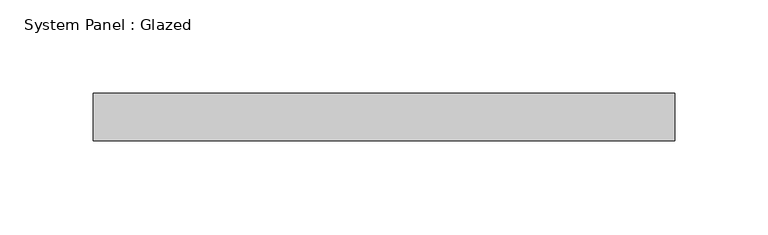
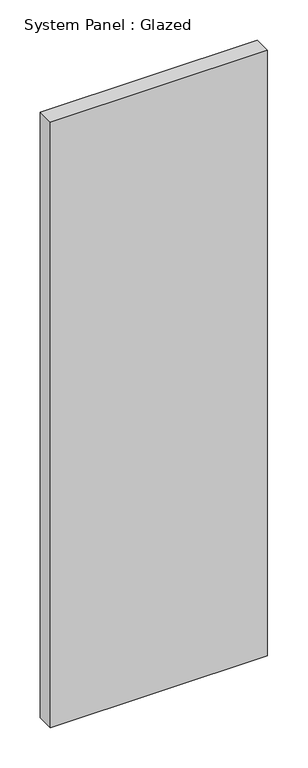
"""IFC4 building model written with IfcOpenShell, lengths in millimetres: plate geometry, System Panel : Glazed."""

from ifc_helpers import new_model, si_unit, origin, origin_with_axes, place, context, project, spatial, polyline, outline, extrude, source, transform, mapped, element, save


def system_panel_glazed_c81023b1(model_context):
    return source(origin(), model_context, "Body", "SweptSolid", [
        extrude(outline(polyline([(155.575, 19.05), (-155.575, 19.05), (-155.575, 44.45), (155.575, 44.45), (155.575, 19.05)])), origin_with_axes(), (0.0, 0.0, 1.0), 918.6333333),
    ])


if __name__ == "__main__":
    model = new_model("IFC4")
    model_context = context("Model", 3, world=origin())
    ifc_project = project(units=[si_unit("LENGTHUNIT", "METRE", prefix="MILLI")], contexts=[model_context])
    site = spatial("IfcSite", under=ifc_project)
    building = spatial("IfcBuilding", under=site)
    placement = place(None, origin())
    system_panel_glazed_shape = system_panel_glazed_c81023b1(model_context)
    element("IfcPlate", 1, ObjectType="System Panel : Glazed", at=placement, inside=building, context=model_context, shape_type="MappedRepresentation", body=[
        mapped(system_panel_glazed_shape, transform((0.0, 0.0, 0.0), x_axis=(1.0, 0.0, 0.0), y_axis=(0.0, 1.0, 0.0), z_axis=(0.0, 0.0, 1.0))),
    ])
    save(model, "model.ifc")

# Revit data of these elements
# Type "System Panel : Glazed"
#   Construction Type Id = "GSP4R"
#   Analytic Construction = "1/8 in Pilkington single glazing"
#   Visual Light Transmittance = 0.9
#   Solar Heat Gain Coefficient = 0.86
#   Heat Transfer Coefficient (U) = 1.18115 BTU/(h·ft²·°F)
# Element 1 (IfcPlate, "System Panel : Glazed")
#   Materials on its faces: "Glass"
# Materials
#   "Glass": class "Glass", colour RGB 0 128 192, transparency 0.75, Description = "Soda Lime Glass", Cost = 0
